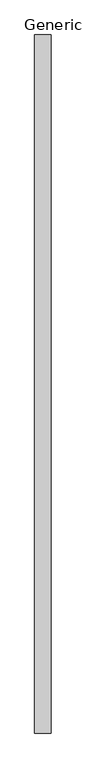
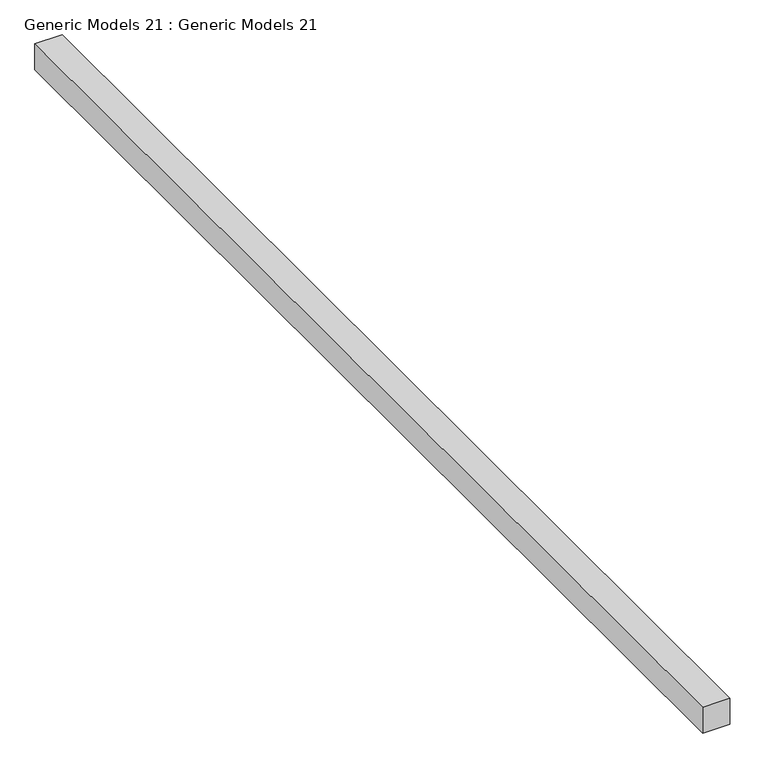
"""IFC4 building model written with IfcOpenShell, lengths in millimetres: proxy geometry, Generic Models 21 : Generic Models 21."""

from ifc_helpers import new_model, si_unit, frame, origin, place, context, project, spatial, polyline, outline, extrude, source, transform, mapped, element, save


def generic_models_21_generic_models_21_4b7ad0a9(model_context):
    return source(origin(), model_context, "Body", "SweptSolid", [
        extrude(outline(polyline([(-15581.438074, -5966.8213044), (-15581.438074, 6941.8014639), (-15276.638074, 6941.8014639), (-15276.638074, -5966.8213044), (-15581.438074, -5966.8213044)])), frame((0.0, 0.0, 9144.0), z_axis=(0.0, 0.0, 1.0), x_axis=(1.0, 0.0, 0.0)), (0.0, 0.0, 1.0), 304.8),
    ])


if __name__ == "__main__":
    model = new_model("IFC4")
    model_context = context("Model", 3, world=origin())
    ifc_project = project(units=[si_unit("LENGTHUNIT", "METRE", prefix="MILLI")], contexts=[model_context])
    site = spatial("IfcSite", under=ifc_project)
    building = spatial("IfcBuilding", under=site)
    placement = place(None, origin())
    generic_models_21_generic_models_21_shape = generic_models_21_generic_models_21_4b7ad0a9(model_context)
    element("IfcBuildingElementProxy", 1, Name="Generic Models 21 : Generic Models 21", ObjectType="Generic Models 21 : Generic Models 21", at=placement, inside=building, context=model_context, shape_type="MappedRepresentation", body=[
        mapped(generic_models_21_generic_models_21_shape, transform((0.0, 0.0, 0.0), x_axis=(1.0, 0.0, 0.0), y_axis=(0.0, 1.0, 0.0), z_axis=(0.0, 0.0, 1.0))),
    ])
    save(model, "model.ifc")
